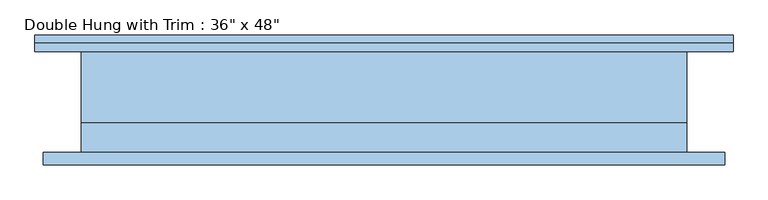
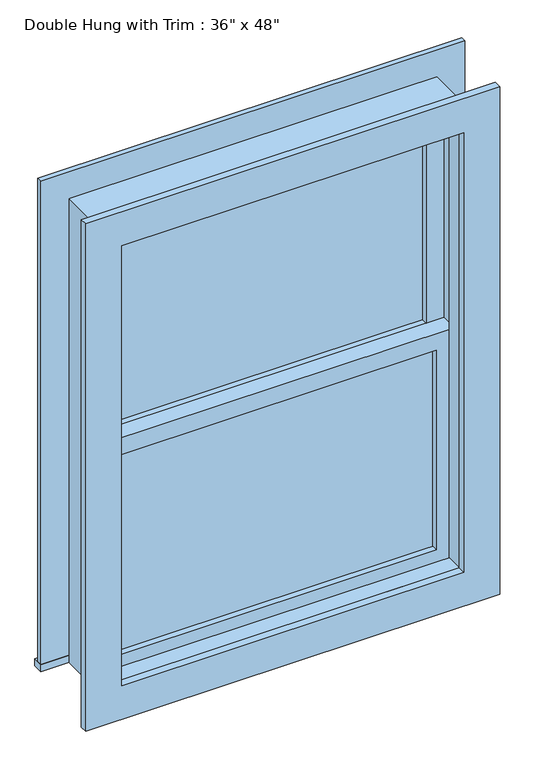
"""IFC4 building model written with IfcOpenShell, lengths in millimetres: window geometry."""

from ifc_helpers import new_model, si_unit, frame, origin, place, context, project, spatial, polyline, outline, extrude, source, transform, mapped, element, save


def window_d24d93a6(model_context):
    return source(origin(), model_context, "Body", "SweptSolid", [
        extrude(outline(polyline([(-393.7, -3.175), (393.7, -3.175), (393.7, -15.875), (-393.7, -15.875), (-393.7, -3.175)])), frame((0.0, 0.0, 977.9), z_axis=(0.0, 0.0, 1.0), x_axis=(1.0, 0.0, 0.0)), (0.0, 0.0, 1.0), 523.875),
        extrude(outline(polyline([(1546.225, -438.15), (933.45, -438.15), (933.45, 438.15), (1546.225, 438.15), (1546.225, -438.15)]), holes=[polyline([(1501.775, -393.7), (1501.775, 393.7), (977.9, 393.7), (977.9, -393.7), (1501.775, -393.7)])]), frame((0.0, -31.75, 0.0), z_axis=(0.0, 1.0, 0.0), x_axis=(0.0, 0.0, 1.0)), (0.0, 0.0, 1.0), 44.45),
        extrude(outline(polyline([(-527.05, 101.6), (527.05, 101.6), (527.05, 76.2), (-527.05, 76.2), (-527.05, 101.6)])), frame((0.0, 0.0, 914.4), z_axis=(0.0, 0.0, 1.0), x_axis=(1.0, 0.0, 0.0)), (0.0, 0.0, 1.0), 19.05),
        extrude(outline(polyline([(2114.55, -438.15), (2114.55, 438.15), (933.45, 438.15), (933.45, 527.05), (2203.45, 527.05), (2203.45, -527.05), (933.45, -527.05), (933.45, -438.15), (2114.55, -438.15)])), frame((0.0, 76.2, 0.0), z_axis=(0.0, 1.0, 0.0), x_axis=(0.0, 0.0, 1.0)), (0.0, 0.0, 1.0), 12.7),
        extrude(outline(polyline([(2190.75, 514.35), (2190.75, -514.35), (857.25, -514.35), (857.25, 514.35), (2190.75, 514.35)]), holes=[polyline([(2101.85, 425.45), (946.15, 425.45), (946.15, -425.45), (2101.85, -425.45), (2101.85, 425.45)])]), frame((0.0, -95.25, 0.0), z_axis=(0.0, 1.0, 0.0), x_axis=(0.0, 0.0, 1.0)), (0.0, 0.0, 1.0), 19.05),
        extrude(outline(polyline([(393.7, 28.575), (-393.7, 28.575), (-393.7, 41.275), (393.7, 41.275), (393.7, 28.575)])), frame((0.0, 0.0, 1546.225), z_axis=(0.0, 0.0, 1.0), x_axis=(1.0, 0.0, 0.0)), (0.0, 0.0, 1.0), 523.875),
        extrude(outline(polyline([(2114.55, -438.15), (1501.775, -438.15), (1501.775, 438.15), (2114.55, 438.15), (2114.55, -438.15)]), holes=[polyline([(2070.1, -393.7), (2070.1, 393.7), (1546.225, 393.7), (1546.225, -393.7), (2070.1, -393.7)])]), frame((0.0, 12.7, 0.0), z_axis=(0.0, 1.0, 0.0), x_axis=(0.0, 0.0, 1.0)), (0.0, 0.0, 1.0), 44.45),
        extrude(outline(polyline([(2133.6, -457.2), (914.4, -457.2), (914.4, 457.2), (2133.6, 457.2), (2133.6, -457.2)]), holes=[polyline([(2101.85, -425.45), (2101.85, 425.45), (946.15, 425.45), (946.15, -425.45), (2101.85, -425.45)])]), frame((0.0, -76.2, 0.0), z_axis=(0.0, 1.0, 0.0), x_axis=(0.0, 0.0, 1.0)), (0.0, 0.0, 1.0), 44.45),
        extrude(outline(polyline([(2133.6, 457.2), (2133.6, -457.2), (914.4, -457.2), (914.4, 457.2), (2133.6, 457.2)]), holes=[polyline([(2114.55, 438.15), (933.45, 438.15), (933.45, -438.15), (2114.55, -438.15), (2114.55, 438.15)])]), frame((0.0, -31.75, 0.0), z_axis=(0.0, 1.0, 0.0), x_axis=(0.0, 0.0, 1.0)), (0.0, 0.0, 1.0), 107.95),
    ])


if __name__ == "__main__":
    model = new_model("IFC4")
    model_context = context("Model", 3, world=origin())
    ifc_project = project(units=[si_unit("LENGTHUNIT", "METRE", prefix="MILLI")], contexts=[model_context])
    site = spatial("IfcSite", under=ifc_project)
    building = spatial("IfcBuilding", under=site)
    placement = place(None, origin())
    window_shape = window_d24d93a6(model_context)
    element("IfcWindow", 1, ObjectType="Double Hung with Trim : 36\" x 48\"", at=placement, inside=building, context=model_context, shape_type="MappedRepresentation", body=[
        mapped(window_shape, transform((0.0, 0.0, 0.0), x_axis=(1.0, 0.0, 0.0), y_axis=(0.0, 1.0, 0.0), z_axis=(0.0, 0.0, 1.0))),
    ])
    save(model, "model.ifc")

# Revit data of these elements
# Type "Double Hung with Trim : 36\" x 48\""
#   Type Mark = "10"
#   Construction Type Id = "GSP4R"
#   Assembly Code = "B2020100"
#   Analytic Construction = "1/8 in Pilkington single glazing"
#   Visual Light Transmittance = 0.9
#   Solar Heat Gain Coefficient = 0.78
#   Heat Transfer Coefficient (U) = 0.6496 BTU/(h·ft²·°F)
#   Height = 4' - 0"
#   Default Sill Height = 3' - 0"
#   Trim Projection - Ext. = 0' - 0 1/2"
#   Trim Projection - Int. = 0' - 0 3/4"
#   Trim Width - Exterior = 0' - 3 1/2"
#   Trim Width - Interior = 0' - 3 1/2"
#   Width = 3' - 0"
#   Window Inset = 0' - 0 3/4"
#   Define Thermal Properties by = 1
#   Glass Pane Material = Glass
#   Sash Material = Sash
#   Trim Exterior Material = Trim
#   Trim Interior Material = Trim
#   Wall Closure = (empty or 0)
# Element 1 (IfcWindow, "Double Hung with Trim : 36\" x 48\"")
#   Materials on its faces: "Sash", "Trim", "Glass"
# Materials
#   "Glass": class "Glass", colour RGB 0 128 192, transparency 0.75, Description = "Soda Lime Glass", Cost = 0
#   "Sash": class "Wood", colour RGB 224 178 126, transparency 0
#   "Trim": class "Wood", colour RGB 224 178 126, transparency 0
